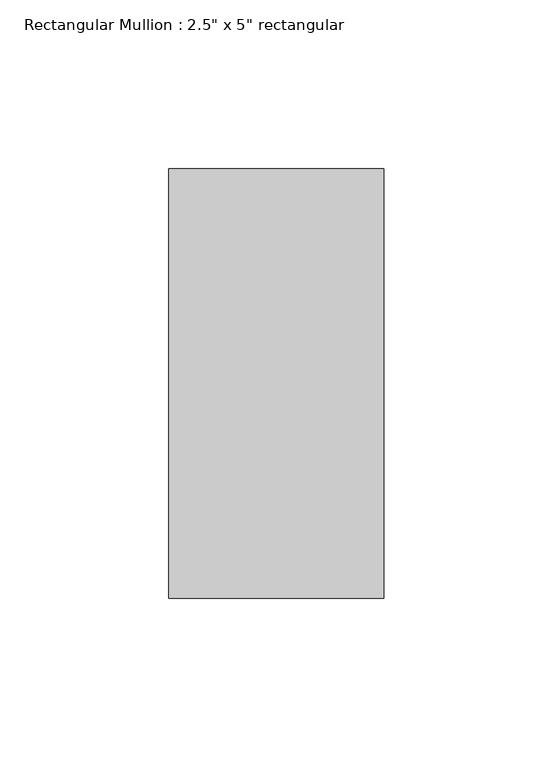
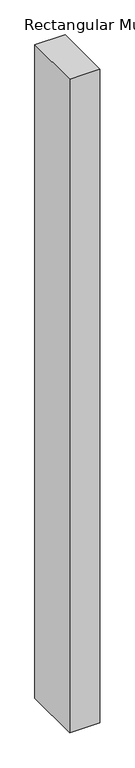
"""IFC4 building model written with IfcOpenShell, lengths in millimetres: member geometry."""

from ifc_helpers import new_model, si_unit, frame, origin, place, context, project, spatial, polyline, outline, extrude, source, transform, mapped, element, save


def member_066849cb(model_context):
    return source(origin(), model_context, "Body", "SweptSolid", [
        extrude(outline(polyline([(0.0, 63.5), (0.0, -63.5), (-63.5, -63.5), (-63.5, 63.5), (0.0, 63.5)])), frame((0.0, 0.0, -1458.3753662), z_axis=(0.0, 0.0, 1.0), x_axis=(1.0, 0.0, 0.0)), (0.0, 0.0, 1.0), 1458.3753662),
    ])


if __name__ == "__main__":
    model = new_model("IFC4")
    model_context = context("Model", 3, world=origin())
    ifc_project = project(units=[si_unit("LENGTHUNIT", "METRE", prefix="MILLI")], contexts=[model_context])
    site = spatial("IfcSite", under=ifc_project)
    building = spatial("IfcBuilding", under=site)
    placement = place(None, origin())
    member_shape = member_066849cb(model_context)
    element("IfcMember", 1, ObjectType="Rectangular Mullion : 2.5\" x 5\" rectangular", at=placement, inside=building, context=model_context, shape_type="MappedRepresentation", body=[
        mapped(member_shape, transform((0.0, 0.0, 0.0), x_axis=(1.0, 0.0, 0.0), y_axis=(0.0, 1.0, 0.0), z_axis=(0.0, 0.0, 1.0))),
    ])
    save(model, "model.ifc")

# Revit data of these elements
# Type "Rectangular Mullion : 2.5\" x 5\" rectangular"
#   built-in parameter 1007304 = 0.416667 (stored number, unit not read)
#   built-in parameter 1007301 = 0.104167 (stored number, unit not read)
#   built-in parameter 1007300 = 0.104167 (stored number, unit not read)
# Element 1 (IfcMember, "Rectangular Mullion : 2.5\" x 5\" rectangular")
#   Materials on its faces: "Aluminum"
# Materials
#   "Aluminum": class "Metal", colour RGB 247 247 247, transparency 0, Description = "Aluminum 6061", Cost = 0
